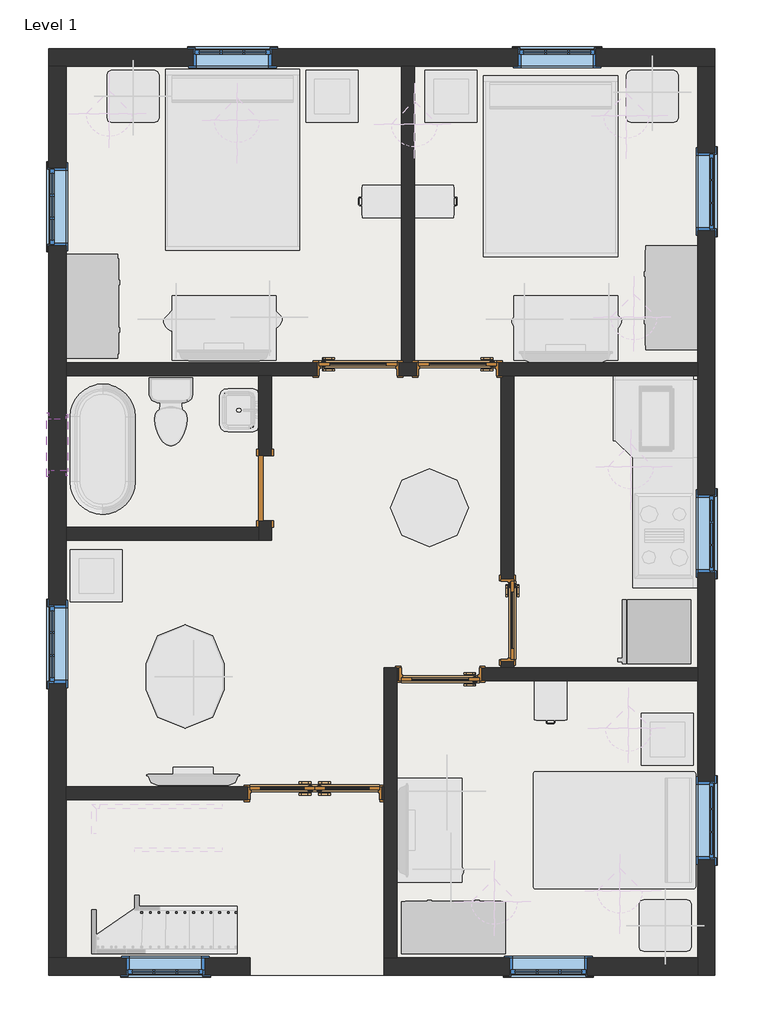
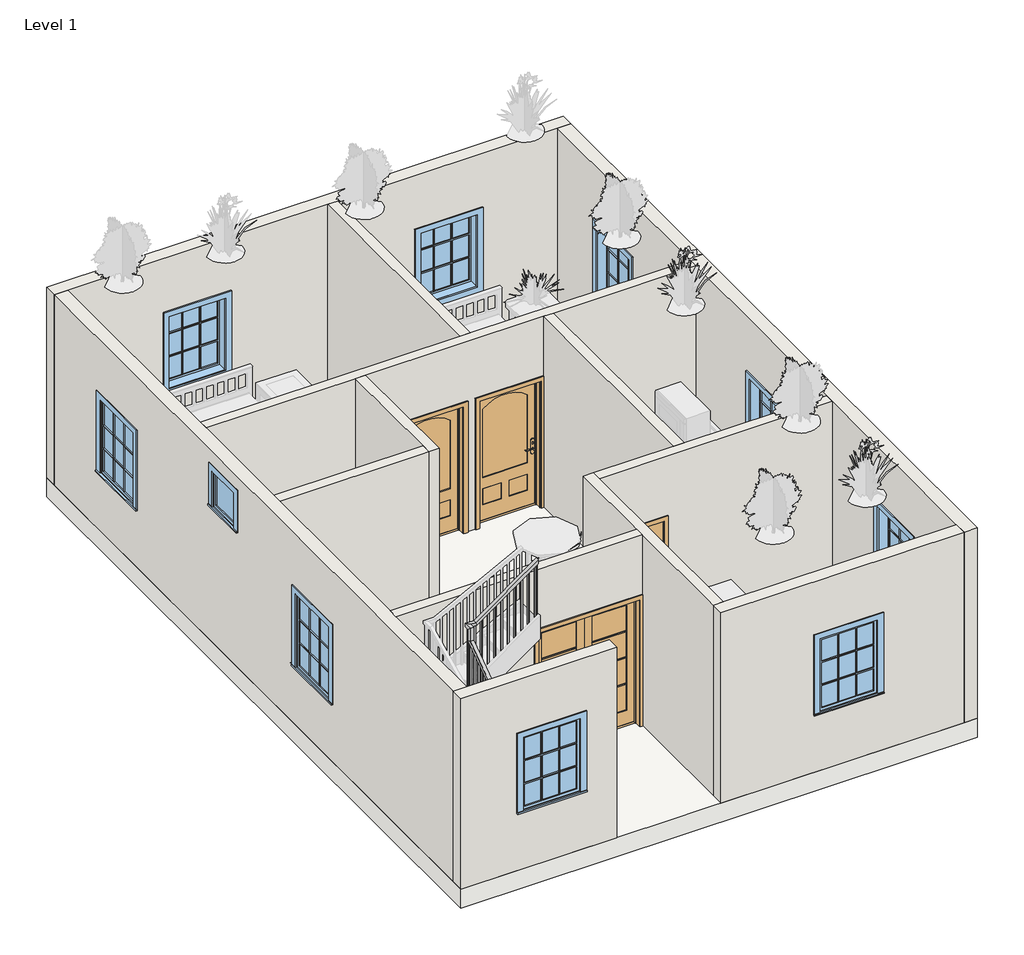
# One storey, part 1 of 2: 13 walls, 10 windows, 6 doors, 1 railing, 1 slab.
"""IFC4 building model written with IfcOpenShell, lengths in millimetres."""

from ifc_helpers import new_model, si_unit, frame, origin, origin_with_axes, place, context, project, spatial, polyline, outline, extrude, faceted_brep, transform, mapped, element, save
from components import door_5d363d20, door_808aeb8e, door_94998e6c, door_255cab33, window_29c06734, window_e41d21a6

model = new_model("IFC4")

# Units and contexts
model_context = context("Model", 3, world=origin())
ifc_project = project(units=[si_unit("LENGTHUNIT", "METRE", prefix="MILLI")], contexts=[model_context])

# Site, building, storey
site = spatial("IfcSite", under=ifc_project)
building = spatial("IfcBuilding", under=site)
storey = spatial("IfcBuildingStorey", under=building, Name="Level 1", Elevation=0.0)

# Doors
placement = place(None, origin())
door_shape = door_5d363d20(model_context)
element("IfcDoor", 1, ObjectType="36\" x 80\"", at=placement, inside=storey, context=model_context, shape_type="MappedRepresentation", body=[
    mapped(door_shape, transform((-9424.8047602, 10392.474435, 0.0), x_axis=(-1.0, 0.0, 0.0), y_axis=(0.0, -1.0, 0.0), z_axis=(0.0, 0.0, 1.0))),
])
element("IfcDoor", 2, ObjectType="36\" x 80\"", at=placement, inside=storey, context=model_context, shape_type="MappedRepresentation", body=[
    mapped(door_shape, transform((-7669.0297602, 7442.899435, 0.0), x_axis=(0.0, 1.0, 0.0), y_axis=(-1.0, 0.0, 0.0), z_axis=(0.0, 0.0, 1.0))),
])
element("IfcDoor", 3, ObjectType="36\" x 80\"", at=placement, inside=storey, context=model_context, shape_type="MappedRepresentation", body=[
    mapped(door_shape, transform((-8459.6047602, 6804.724435, 0.0), x_axis=(1.0, 0.0, 0.0), y_axis=(0.0, 1.0, 0.0), z_axis=(0.0, 0.0, 1.0))),
])
door_2_shape = door_808aeb8e(model_context)
element("IfcDoor", 4, ObjectType="36\" x 80\"", at=placement, inside=storey, context=model_context, shape_type="MappedRepresentation", body=[
    mapped(door_2_shape, transform((-8256.4047602, 10392.474435, 0.0), x_axis=(1.0, 0.0, 0.0), y_axis=(0.0, 1.0, 0.0), z_axis=(0.0, 0.0, 1.0))),
])
door_3_shape = door_94998e6c(model_context)
element("IfcDoor", 5, ObjectType="Door-Exterior-Double-Full Glass-Wood_Clad : 60\" x 80\"", at=placement, inside=storey, context=model_context, shape_type="MappedRepresentation", body=[
    mapped(door_3_shape, transform((-9932.8047602, 5414.074435, 0.0), x_axis=(1.0, 0.0, 0.0), y_axis=(0.0, 1.0, 0.0), z_axis=(0.0, 0.0, 1.0))),
])
door_4_shape = door_255cab33(model_context)
element("IfcDoor", 6, ObjectType="Single-Flush : 30\" x 80\"", at=placement, inside=storey, context=model_context, shape_type="MappedRepresentation", body=[
    mapped(door_4_shape, transform((-10517.0047602, 8992.299435, 0.0), x_axis=(0.0, -1.0, 0.0), y_axis=(1.0, 0.0, 0.0), z_axis=(0.0, 0.0, 1.0))),
])

# Railing
element("IfcRailing", 7, ObjectType="Handrail - Rectangular", at=placement, inside=storey, context=model_context, shape_type="SolidModel", body=[
    faceted_brep([(-10847.2047602, 3988.499435, 1381.9082396), (-10847.2047602, 3988.499435, 1318.3782167), (-10847.2047602, 4039.299435, 1318.3782167), (-10847.2047602, 4039.299435, 1381.9082396), (-11968.5364521, 3988.499435, 2224.0110577), (-12019.3364521, 3988.499435, 2198.6310519), (-12019.3364521, 4039.299435, 2198.6310519), (-11968.5364521, 4039.299435, 2224.0110577), (-11968.5364521, 3988.499435, 2365.3316897), (-12019.3364521, 3988.499435, 2314.5316897), (-12019.3364521, 4039.299435, 2314.5316897), (-11968.5364521, 4039.299435, 2365.3316897), (-12095.5364521, 3988.499435, 2365.3316897), (-12095.5364521, 3988.499435, 2314.5316897), (-12044.7364521, 4039.299435, 2314.5316897), (-12044.7364521, 4039.299435, 2365.3316897), (-12095.5364521, 4115.499435, 2365.3316897), (-12095.5364521, 4131.3621783, 2314.5316897), (-12044.7364521, 4131.3621783, 2314.5316897), (-12044.7364521, 4115.499435, 2365.3316897), (-12095.5364521, 4699.699435, 2769.5924376), (-12095.5364521, 4750.499435, 2742.9686812), (-12044.7364521, 4750.499435, 2742.9686812), (-12044.7364521, 4699.699435, 2769.5924376), (-12095.5364521, 4699.699435, 2979.2954752), (-12095.5364521, 4750.499435, 2928.4954752), (-12044.7364521, 4750.499435, 2928.4954752), (-12044.7364521, 4699.699435, 2979.2954752), (-12095.5364521, 4826.699435, 2979.2954752), (-12095.5364521, 4826.699435, 2928.4954752), (-12044.7364521, 4775.899435, 2928.4954752), (-12044.7364521, 4775.899435, 2979.2954752), (-11968.5364521, 4826.699435, 2979.2954752), (-11952.2655241, 4826.699435, 2928.4954752), (-11952.2655241, 4775.899435, 2928.4954752), (-11968.5364521, 4775.899435, 2979.2954752), (-11023.5532442, 4826.699435, 3653.8404346), (-11023.5532442, 4775.899435, 3653.8404346), (-11023.5532442, 4775.899435, 3591.4259716), (-11023.5532442, 4826.699435, 3591.4259716)], [[[0, 1, 2, 3]], [[1, 0, 4, 5]], [[2, 1, 5, 6]], [[3, 2, 6, 7]], [[0, 3, 7, 4]], [[5, 4, 8, 9]], [[6, 5, 9, 10]], [[7, 6, 10, 11]], [[4, 7, 11, 8]], [[9, 8, 12, 13]], [[10, 9, 13, 14]], [[11, 10, 14, 15]], [[8, 11, 15, 12]], [[13, 12, 16, 17]], [[14, 13, 17, 18]], [[15, 14, 18, 19]], [[12, 15, 19, 16]], [[17, 16, 20, 21]], [[18, 17, 21, 22]], [[19, 18, 22, 23]], [[16, 19, 23, 20]], [[21, 20, 24, 25]], [[22, 21, 25, 26]], [[23, 22, 26, 27]], [[20, 23, 27, 24]], [[25, 24, 28, 29]], [[26, 25, 29, 30]], [[27, 26, 30, 31]], [[24, 27, 31, 28]], [[29, 28, 32, 33]], [[30, 29, 33, 34]], [[31, 30, 34, 35]], [[28, 31, 35, 32]], [[36, 37, 38, 39]], [[33, 32, 36, 39]], [[34, 33, 39, 38]], [[35, 34, 38, 37]], [[32, 35, 37, 36]]]),
    extrude(outline(polyline([(3576.3942675, -11044.6114521), (3562.796056, -11063.6614521), (2540.0, -11063.6614521), (2540.0, -11044.6114521), (3576.3942675, -11044.6114521)])), frame((0.0, 4791.774435, 0.0), z_axis=(0.0, 1.0, 0.0), x_axis=(0.0, 0.0, 1.0)), (0.0, 0.0, 1.0), 19.05),
    extrude(outline(polyline([(3503.8704731, -11146.2114521), (3490.2722616, -11165.2614521), (2540.0, -11165.2614521), (2540.0, -11146.2114521), (3503.8704731, -11146.2114521)])), frame((0.0, 4791.774435, 0.0), z_axis=(0.0, 1.0, 0.0), x_axis=(0.0, 0.0, 1.0)), (0.0, 0.0, 1.0), 19.05),
    extrude(outline(polyline([(3431.3466787, -11247.8114521), (3417.7484672, -11266.8614521), (2540.0, -11266.8614521), (2540.0, -11247.8114521), (3431.3466787, -11247.8114521)])), frame((0.0, 4791.774435, 0.0), z_axis=(0.0, 1.0, 0.0), x_axis=(0.0, 0.0, 1.0)), (0.0, 0.0, 1.0), 19.05),
    extrude(outline(polyline([(3358.8228843, -11349.4114521), (3345.2246729, -11368.4614521), (2370.6666667, -11368.4614521), (2370.6666667, -11349.4114521), (3358.8228843, -11349.4114521)])), frame((0.0, 4791.774435, 0.0), z_axis=(0.0, 1.0, 0.0), x_axis=(0.0, 0.0, 1.0)), (0.0, 0.0, 1.0), 19.05),
    extrude(outline(polyline([(3286.2990899, -11451.0114521), (3272.7008785, -11470.0614521), (2370.6666667, -11470.0614521), (2370.6666667, -11451.0114521), (3286.2990899, -11451.0114521)])), frame((0.0, 4791.774435, 0.0), z_axis=(0.0, 1.0, 0.0), x_axis=(0.0, 0.0, 1.0)), (0.0, 0.0, 1.0), 19.05),
    extrude(outline(polyline([(3213.7752955, -11552.6114521), (3200.1770841, -11571.6614521), (2370.6666667, -11571.6614521), (2370.6666667, -11552.6114521), (3213.7752955, -11552.6114521)])), frame((0.0, 4791.774435, 0.0), z_axis=(0.0, 1.0, 0.0), x_axis=(0.0, 0.0, 1.0)), (0.0, 0.0, 1.0), 19.05),
    extrude(outline(polyline([(3141.2515011, -11654.2114521), (3127.6532897, -11673.2614521), (2201.3333333, -11673.2614521), (2201.3333333, -11654.2114521), (3141.2515011, -11654.2114521)])), frame((0.0, 4791.774435, 0.0), z_axis=(0.0, 1.0, 0.0), x_axis=(0.0, 0.0, 1.0)), (0.0, 0.0, 1.0), 19.05),
    extrude(outline(polyline([(3068.7277067, -11755.8114521), (3055.1294953, -11774.8614521), (2201.3333333, -11774.8614521), (2201.3333333, -11755.8114521), (3068.7277067, -11755.8114521)])), frame((0.0, 4791.774435, 0.0), z_axis=(0.0, 1.0, 0.0), x_axis=(0.0, 0.0, 1.0)), (0.0, 0.0, 1.0), 19.05),
    extrude(outline(polyline([(2996.2039123, -11857.4114521), (2982.6057009, -11876.4614521), (2032.0, -11876.4614521), (2032.0, -11857.4114521), (2996.2039123, -11857.4114521)])), frame((0.0, 4791.774435, 0.0), z_axis=(0.0, 1.0, 0.0), x_axis=(0.0, 0.0, 1.0)), (0.0, 0.0, 1.0), 19.05),
    extrude(outline(polyline([(-11978.0614521, 4791.774435), (-11978.0614521, 4810.824435), (-11959.0114521, 4810.824435), (-11959.0114521, 4791.774435), (-11978.0614521, 4791.774435)])), frame((0.0, 0.0, 2032.0), z_axis=(0.0, 0.0, 1.0), x_axis=(1.0, 0.0, 0.0)), (0.0, 0.0, 1.0), 896.4954752),
    extrude(outline(polyline([(4719.3935773, 2721.4437287), (4738.4435773, 2734.6261443), (4738.4435773, 1862.6666667), (4719.3935773, 1862.6666667), (4719.3935773, 2721.4437287)])), frame((-12079.6614521, 0.0, 0.0), z_axis=(1.0, 0.0, 0.0), x_axis=(0.0, 1.0, 0.0)), (0.0, 0.0, 1.0), 19.05),
    extrude(outline(polyline([(4617.7935773, 2651.1375116), (4636.8435773, 2664.3199273), (4636.8435773, 1693.3333333), (4617.7935773, 1693.3333333), (4617.7935773, 2651.1375116)])), frame((-12079.6614521, 0.0, 0.0), z_axis=(1.0, 0.0, 0.0), x_axis=(0.0, 1.0, 0.0)), (0.0, 0.0, 1.0), 19.05),
    extrude(outline(polyline([(4516.1935773, 2580.8312946), (4535.2435773, 2594.0137103), (4535.2435773, 1693.3333333), (4516.1935773, 1693.3333333), (4516.1935773, 2580.8312946)])), frame((-12079.6614521, 0.0, 0.0), z_axis=(1.0, 0.0, 0.0), x_axis=(0.0, 1.0, 0.0)), (0.0, 0.0, 1.0), 19.05),
    extrude(outline(polyline([(4414.5935773, 2510.5250776), (4433.6435773, 2523.7074933), (4433.6435773, 1524.0), (4414.5935773, 1524.0), (4414.5935773, 2510.5250776)])), frame((-12079.6614521, 0.0, 0.0), z_axis=(1.0, 0.0, 0.0), x_axis=(0.0, 1.0, 0.0)), (0.0, 0.0, 1.0), 19.05),
    extrude(outline(polyline([(4312.9935773, 2440.2188606), (4332.0435773, 2453.4012762), (4332.0435773, 1524.0), (4312.9935773, 1524.0), (4312.9935773, 2440.2188606)])), frame((-12079.6614521, 0.0, 0.0), z_axis=(1.0, 0.0, 0.0), x_axis=(0.0, 1.0, 0.0)), (0.0, 0.0, 1.0), 19.05),
    extrude(outline(polyline([(4211.3935773, 2369.9126435), (4230.4435773, 2383.0950592), (4230.4435773, 1524.0), (4211.3935773, 1524.0), (4211.3935773, 2369.9126435)])), frame((-12079.6614521, 0.0, 0.0), z_axis=(1.0, 0.0, 0.0), x_axis=(0.0, 1.0, 0.0)), (0.0, 0.0, 1.0), 19.05),
    extrude(outline(polyline([(4109.7935773, 2299.6064265), (4128.8435773, 2312.7888422), (4128.8435773, 1354.6666667), (4109.7935773, 1354.6666667), (4109.7935773, 2299.6064265)])), frame((-12079.6614521, 0.0, 0.0), z_axis=(1.0, 0.0, 0.0), x_axis=(0.0, 1.0, 0.0)), (0.0, 0.0, 1.0), 19.05),
    extrude(outline(polyline([(-12056.8797602, 4023.424435), (-12056.8797602, 4004.374435), (-12075.9297602, 4004.374435), (-12075.9297602, 4023.424435), (-12056.8797602, 4023.424435)])), frame((0.0, 0.0, 1354.6666667), z_axis=(0.0, 0.0, 1.0), x_axis=(1.0, 0.0, 0.0)), (0.0, 0.0, 1.0), 959.865023),
    extrude(outline(polyline([(2150.5254636, -11955.2797602), (2164.83172, -11974.3297602), (1185.3333333, -11974.3297602), (1185.3333333, -11955.2797602), (2150.5254636, -11955.2797602)])), frame((0.0, 4004.374435, 0.0), z_axis=(0.0, 1.0, 0.0), x_axis=(0.0, 0.0, 1.0)), (0.0, 0.0, 1.0), 19.05),
    extrude(outline(polyline([(2074.2254295, -11853.6797602), (2088.5316859, -11872.7297602), (1016.0, -11872.7297602), (1016.0, -11853.6797602), (2074.2254295, -11853.6797602)])), frame((0.0, 4004.374435, 0.0), z_axis=(0.0, 1.0, 0.0), x_axis=(0.0, 0.0, 1.0)), (0.0, 0.0, 1.0), 19.05),
    extrude(outline(polyline([(1997.9253954, -11752.0797602), (2012.2316518, -11771.1297602), (1016.0, -11771.1297602), (1016.0, -11752.0797602), (1997.9253954, -11752.0797602)])), frame((0.0, 4004.374435, 0.0), z_axis=(0.0, 1.0, 0.0), x_axis=(0.0, 0.0, 1.0)), (0.0, 0.0, 1.0), 19.05),
    extrude(outline(polyline([(1921.6253613, -11650.4797602), (1935.9316177, -11669.5297602), (846.6666667, -11669.5297602), (846.6666667, -11650.4797602), (1921.6253613, -11650.4797602)])), frame((0.0, 4004.374435, 0.0), z_axis=(0.0, 1.0, 0.0), x_axis=(0.0, 0.0, 1.0)), (0.0, 0.0, 1.0), 19.05),
    extrude(outline(polyline([(1845.3253272, -11548.8797602), (1859.6315836, -11567.9297602), (846.6666667, -11567.9297602), (846.6666667, -11548.8797602), (1845.3253272, -11548.8797602)])), frame((0.0, 4004.374435, 0.0), z_axis=(0.0, 1.0, 0.0), x_axis=(0.0, 0.0, 1.0)), (0.0, 0.0, 1.0), 19.05),
    extrude(outline(polyline([(1769.0252931, -11447.2797602), (1783.3315495, -11466.3297602), (846.6666667, -11466.3297602), (846.6666667, -11447.2797602), (1769.0252931, -11447.2797602)])), frame((0.0, 4004.374435, 0.0), z_axis=(0.0, 1.0, 0.0), x_axis=(0.0, 0.0, 1.0)), (0.0, 0.0, 1.0), 19.05),
    extrude(outline(polyline([(1692.725259, -11345.6797602), (1707.0315154, -11364.7297602), (677.3333333, -11364.7297602), (677.3333333, -11345.6797602), (1692.725259, -11345.6797602)])), frame((0.0, 4004.374435, 0.0), z_axis=(0.0, 1.0, 0.0), x_axis=(0.0, 0.0, 1.0)), (0.0, 0.0, 1.0), 19.05),
    extrude(outline(polyline([(1616.4252249, -11244.0797602), (1630.7314813, -11263.1297602), (677.3333333, -11263.1297602), (677.3333333, -11244.0797602), (1616.4252249, -11244.0797602)])), frame((0.0, 4004.374435, 0.0), z_axis=(0.0, 1.0, 0.0), x_axis=(0.0, 0.0, 1.0)), (0.0, 0.0, 1.0), 19.05),
    extrude(outline(polyline([(1540.1251908, -11142.4797602), (1554.4314472, -11161.5297602), (677.3333333, -11161.5297602), (677.3333333, -11142.4797602), (1540.1251908, -11142.4797602)])), frame((0.0, 4004.374435, 0.0), z_axis=(0.0, 1.0, 0.0), x_axis=(0.0, 0.0, 1.0)), (0.0, 0.0, 1.0), 19.05),
    extrude(outline(polyline([(1463.8251567, -11040.8797602), (1478.1314131, -11059.9297602), (508.0, -11059.9297602), (508.0, -11040.8797602), (1463.8251567, -11040.8797602)])), frame((0.0, 4004.374435, 0.0), z_axis=(0.0, 1.0, 0.0), x_axis=(0.0, 0.0, 1.0)), (0.0, 0.0, 1.0), 19.05),
    extrude(outline(polyline([(1387.5251226, -10939.2797602), (1401.831379, -10958.3297602), (508.0, -10958.3297602), (508.0, -10939.2797602), (1387.5251226, -10939.2797602)])), frame((0.0, 4004.374435, 0.0), z_axis=(0.0, 1.0, 0.0), x_axis=(0.0, 0.0, 1.0)), (0.0, 0.0, 1.0), 19.05),
    extrude(outline(polyline([(-12079.6614521, 4791.774435), (-12079.6614521, 4810.824435), (-12060.6114521, 4810.824435), (-12060.6114521, 4791.774435), (-12079.6614521, 4791.774435)])), frame((0.0, 0.0, 1862.6666667), z_axis=(0.0, 0.0, 1.0), x_axis=(1.0, 0.0, 0.0)), (0.0, 0.0, 1.0), 1065.8288085),
    extrude(outline(polyline([(-12060.6114521, 4008.1935773), (-12079.6614521, 4008.1935773), (-12079.6614521, 4027.2435773), (-12060.6114521, 4027.2435773), (-12060.6114521, 4008.1935773)])), frame((0.0, 0.0, 1354.6666667), z_axis=(0.0, 0.0, 1.0), x_axis=(1.0, 0.0, 0.0)), (0.0, 0.0, 1.0), 959.865023),
    extrude(outline(polyline([(-12060.6114521, 4023.424435), (-12060.6114521, 4004.374435), (-12079.6614521, 4004.374435), (-12079.6614521, 4023.424435), (-12060.6114521, 4023.424435)])), frame((0.0, 0.0, 1354.6666667), z_axis=(0.0, 0.0, 1.0), x_axis=(1.0, 0.0, 0.0)), (0.0, 0.0, 1.0), 959.865023),
    extrude(outline(polyline([(-12057.0923258, 4023.424435), (-12057.0923258, 4004.374435), (-12076.1423258, 4004.374435), (-12076.1423258, 4023.424435), (-12057.0923258, 4023.424435)])), frame((0.0, 0.0, 1354.6666667), z_axis=(0.0, 0.0, 1.0), x_axis=(1.0, 0.0, 0.0)), (0.0, 0.0, 1.0), 959.865023),
    extrude(outline(polyline([(3591.4259716, -11023.5532442), (3577.8277602, -11042.6032442), (2540.0, -11042.6032442), (2540.0, -11023.5532442), (3591.4259716, -11023.5532442)])), frame((0.0, 4791.774435, 0.0), z_axis=(0.0, 1.0, 0.0), x_axis=(0.0, 0.0, 1.0)), (0.0, 0.0, 1.0), 19.05),
    extrude(outline(polyline([(1318.3782167, -10847.2047602), (1332.6844731, -10866.2547602), (508.0, -10866.2547602), (508.0, -10847.2047602), (1318.3782167, -10847.2047602)])), frame((0.0, 4004.374435, 0.0), z_axis=(0.0, 1.0, 0.0), x_axis=(0.0, 0.0, 1.0)), (0.0, 0.0, 1.0), 19.05),
])

# Slab
element("IfcSlab", 8, ObjectType="Generic - 12\"", at=placement, inside=storey, context=model_context, shape_type="SweptSolid", body=[
    extrude(outline(polyline([(-5233.8047602, 14148.499435), (-5233.8047602, 3277.299435), (-13057.0047602, 3277.299435), (-13057.0047602, 14148.499435), (-5233.8047602, 14148.499435)])), frame((0.0, 0.0, -304.8), z_axis=(0.0, 0.0, 1.0), x_axis=(1.0, 0.0, 0.0)), (0.0, 0.0, 1.0), 304.8),
])

# Walls
element("IfcWall", 9, ObjectType="Generic - 8\"", at=placement, inside=storey, context=model_context, shape_type="Brep", body=[
    faceted_brep([(-13057.0047602, 13945.299435, 0.0), (-12853.8047602, 13945.299435, 0.0), (-8916.8047602, 13945.299435, 0.0), (-8764.4047602, 13945.299435, 0.0), (-5437.0047602, 13945.299435, 0.0), (-5233.8047602, 13945.299435, 0.0), (-5233.8047602, 13945.299435, 3048.0), (-5437.0047602, 13945.299435, 3048.0), (-8764.4047602, 13945.299435, 3048.0), (-8916.8047602, 13945.299435, 3048.0), (-12853.8047602, 13945.299435, 3048.0), (-13057.0047602, 13945.299435, 3048.0), (-10440.8047602, 13945.299435, 2133.6), (-10440.8047602, 13945.299435, 914.4), (-11355.2047602, 13945.299435, 914.4), (-11355.2047602, 13945.299435, 2133.6), (-6630.8047602, 13945.299435, 2133.6), (-6630.8047602, 13945.299435, 914.4), (-7545.2047602, 13945.299435, 914.4), (-7545.2047602, 13945.299435, 2133.6), (-13057.0047602, 14148.499435, 0.0), (-13057.0047602, 14148.499435, 3048.0), (-5233.8047602, 14148.499435, 3048.0), (-5233.8047602, 14148.499435, 0.0), (-10440.8047602, 14148.499435, 2133.6), (-11355.2047602, 14148.499435, 2133.6), (-11355.2047602, 14148.499435, 914.4), (-10440.8047602, 14148.499435, 914.4), (-6630.8047602, 14148.499435, 2133.6), (-7545.2047602, 14148.499435, 2133.6), (-7545.2047602, 14148.499435, 914.4), (-6630.8047602, 14148.499435, 914.4)], [[[0, 1, 2, 3, 4, 5, 6, 7, 8, 9, 10, 11], [12, 13, 14, 15], [16, 17, 18, 19]], [[20, 21, 22, 23], [24, 25, 26, 27], [28, 29, 30, 31]], [[5, 4, 3, 2, 1, 0, 20, 23]], [[6, 5, 23, 22]], [[0, 11, 21, 20]], [[13, 12, 24, 27]], [[14, 13, 27, 26]], [[15, 14, 26, 25]], [[12, 15, 25, 24]], [[17, 16, 28, 31]], [[18, 17, 31, 30]], [[19, 18, 30, 29]], [[16, 19, 29, 28]], [[11, 10, 9, 8, 7, 6, 22, 21]]]),
])
element("IfcWall", 10, ObjectType="Generic - 8\"", at=placement, inside=storey, context=model_context, shape_type="Brep", body=[
    faceted_brep([(-5437.0047602, 13945.299435, 0.0), (-5437.0047602, 10465.499435, 0.0), (-5437.0047602, 10313.099435, 0.0), (-5437.0047602, 6884.099435, 0.0), (-5437.0047602, 6731.699435, 0.0), (-5437.0047602, 3480.499435, 0.0), (-5437.0047602, 3277.299435, 0.0), (-5437.0047602, 3277.299435, 3048.0), (-5437.0047602, 3480.499435, 3048.0), (-5437.0047602, 6731.699435, 3048.0), (-5437.0047602, 6884.099435, 3048.0), (-5437.0047602, 10313.099435, 3048.0), (-5437.0047602, 10465.499435, 3048.0), (-5437.0047602, 13945.299435, 3048.0), (-5437.0047602, 12014.899435, 2133.6), (-5437.0047602, 12014.899435, 914.4), (-5437.0047602, 12929.299435, 914.4), (-5437.0047602, 12929.299435, 2133.6), (-5437.0047602, 8001.699435, 2133.6), (-5437.0047602, 8001.699435, 914.4), (-5437.0047602, 8916.099435, 914.4), (-5437.0047602, 8916.099435, 2133.6), (-5437.0047602, 4636.199435, 2133.6), (-5437.0047602, 4636.199435, 914.4), (-5437.0047602, 5550.599435, 914.4), (-5437.0047602, 5550.599435, 2133.6), (-5233.8047602, 13945.299435, 0.0), (-5233.8047602, 13945.299435, 3048.0), (-5233.8047602, 3277.299435, 3048.0), (-5233.8047602, 3277.299435, 0.0), (-5233.8047602, 12014.899435, 2133.6), (-5233.8047602, 12929.299435, 2133.6), (-5233.8047602, 12929.299435, 914.4), (-5233.8047602, 12014.899435, 914.4), (-5233.8047602, 8001.699435, 2133.6), (-5233.8047602, 8916.099435, 2133.6), (-5233.8047602, 8916.099435, 914.4), (-5233.8047602, 8001.699435, 914.4), (-5233.8047602, 4636.199435, 2133.6), (-5233.8047602, 5550.599435, 2133.6), (-5233.8047602, 5550.599435, 914.4), (-5233.8047602, 4636.199435, 914.4)], [[[0, 1, 2, 3, 4, 5, 6, 7, 8, 9, 10, 11, 12, 13], [14, 15, 16, 17], [18, 19, 20, 21], [22, 23, 24, 25]], [[26, 27, 28, 29], [30, 31, 32, 33], [34, 35, 36, 37], [38, 39, 40, 41]], [[6, 5, 4, 3, 2, 1, 0, 26, 29]], [[0, 13, 27, 26]], [[7, 6, 29, 28]], [[15, 14, 30, 33]], [[16, 15, 33, 32]], [[17, 16, 32, 31]], [[14, 17, 31, 30]], [[19, 18, 34, 37]], [[20, 19, 37, 36]], [[21, 20, 36, 35]], [[18, 21, 35, 34]], [[23, 22, 38, 41]], [[24, 23, 41, 40]], [[25, 24, 40, 39]], [[22, 25, 39, 38]], [[13, 12, 11, 10, 9, 8, 7, 28, 27]]]),
])
element("IfcWall", 11, ObjectType="Generic - 8\"", at=placement, inside=storey, context=model_context, shape_type="Brep", body=[
    faceted_brep([(-5437.0047602, 3480.499435, 0.0), (-8967.6047602, 3480.499435, 0.0), (-9120.0047602, 3480.499435, 0.0), (-9120.0047602, 3480.499435, 3048.0), (-8967.6047602, 3480.499435, 3048.0), (-5437.0047602, 3480.499435, 3048.0), (-7646.8047602, 3480.499435, 2133.6), (-7646.8047602, 3480.499435, 914.4), (-6732.4047602, 3480.499435, 914.4), (-6732.4047602, 3480.499435, 2133.6), (-5437.0047602, 3277.299435, 0.0), (-5437.0047602, 3277.299435, 3048.0), (-9120.0047602, 3277.299435, 3048.0), (-9120.0047602, 3277.299435, 0.0), (-7646.8047602, 3277.299435, 2133.6), (-6732.4047602, 3277.299435, 2133.6), (-6732.4047602, 3277.299435, 914.4), (-7646.8047602, 3277.299435, 914.4)], [[[0, 1, 2, 3, 4, 5], [6, 7, 8, 9]], [[10, 11, 12, 13], [14, 15, 16, 17]], [[2, 1, 0, 10, 13]], [[0, 5, 11, 10]], [[7, 6, 14, 17]], [[8, 7, 17, 16]], [[9, 8, 16, 15]], [[6, 9, 15, 14]], [[3, 2, 13, 12]], [[5, 4, 3, 12, 11]]]),
])
element("IfcWall", 12, ObjectType="Generic - 8\"", at=placement, inside=storey, context=model_context, shape_type="Brep", body=[
    faceted_brep([(-12853.8047602, 3480.499435, 0.0), (-12853.8047602, 5334.699435, 0.0), (-12853.8047602, 5487.099435, 0.0), (-12853.8047602, 8382.699435, 0.0), (-12853.8047602, 8535.099435, 0.0), (-12853.8047602, 10313.099435, 0.0), (-12853.8047602, 10465.499435, 0.0), (-12853.8047602, 13945.299435, 0.0), (-12853.8047602, 13945.299435, 3048.0), (-12853.8047602, 10465.499435, 3048.0), (-12853.8047602, 10313.099435, 3048.0), (-12853.8047602, 8535.099435, 3048.0), (-12853.8047602, 8382.699435, 3048.0), (-12853.8047602, 5487.099435, 3048.0), (-12853.8047602, 5334.699435, 3048.0), (-12853.8047602, 3480.499435, 3048.0), (-12853.8047602, 12751.499435, 2133.6), (-12853.8047602, 12751.499435, 914.4), (-12853.8047602, 11837.099435, 914.4), (-12853.8047602, 11837.099435, 2133.6), (-12853.8047602, 7620.699435, 2133.6), (-12853.8047602, 7620.699435, 914.4), (-12853.8047602, 6706.299435, 914.4), (-12853.8047602, 6706.299435, 2133.6), (-12853.8047602, 9805.099435, 2768.6), (-12853.8047602, 9805.099435, 2159.0), (-12853.8047602, 9195.499435, 2159.0), (-12853.8047602, 9195.499435, 2768.6), (-13057.0047602, 3480.499435, 0.0), (-13057.0047602, 3480.499435, 3048.0), (-13057.0047602, 13945.299435, 3048.0), (-13057.0047602, 13945.299435, 0.0), (-13057.0047602, 12751.499435, 2133.6), (-13057.0047602, 11837.099435, 2133.6), (-13057.0047602, 11837.099435, 914.4), (-13057.0047602, 12751.499435, 914.4), (-13057.0047602, 7620.699435, 2133.6), (-13057.0047602, 6706.299435, 2133.6), (-13057.0047602, 6706.299435, 914.4), (-13057.0047602, 7620.699435, 914.4), (-13057.0047602, 9805.099435, 2768.6), (-13057.0047602, 9195.499435, 2768.6), (-13057.0047602, 9195.499435, 2159.0), (-13057.0047602, 9805.099435, 2159.0)], [[[0, 1, 2, 3, 4, 5, 6, 7, 8, 9, 10, 11, 12, 13, 14, 15], [16, 17, 18, 19], [20, 21, 22, 23], [24, 25, 26, 27]], [[28, 29, 30, 31], [32, 33, 34, 35], [36, 37, 38, 39], [40, 41, 42, 43]], [[7, 6, 5, 4, 3, 2, 1, 0, 28, 31]], [[8, 7, 31, 30]], [[0, 15, 29, 28]], [[17, 16, 32, 35]], [[18, 17, 35, 34]], [[19, 18, 34, 33]], [[16, 19, 33, 32]], [[21, 20, 36, 39]], [[22, 21, 39, 38]], [[23, 22, 38, 37]], [[20, 23, 37, 36]], [[25, 24, 40, 43]], [[26, 25, 43, 42]], [[27, 26, 42, 41]], [[24, 27, 41, 40]], [[15, 14, 13, 12, 11, 10, 9, 8, 30, 29]]]),
])
element("IfcWall", 13, ObjectType="Generic - 8\"", at=placement, inside=storey, context=model_context, shape_type="Brep", body=[
    faceted_brep([(-10694.8047602, 3480.499435, 0.0), (-12853.8047602, 3480.499435, 0.0), (-13057.0047602, 3480.499435, 0.0), (-13057.0047602, 3480.499435, 3048.0), (-12853.8047602, 3480.499435, 3048.0), (-10694.8047602, 3480.499435, 3048.0), (-12142.6047602, 3480.499435, 2133.6), (-12142.6047602, 3480.499435, 914.4), (-11228.2047602, 3480.499435, 914.4), (-11228.2047602, 3480.499435, 2133.6), (-10694.8047602, 3277.299435, 0.0), (-10694.8047602, 3277.299435, 3048.0), (-13057.0047602, 3277.299435, 3048.0), (-13057.0047602, 3277.299435, 0.0), (-12142.6047602, 3277.299435, 2133.6), (-11228.2047602, 3277.299435, 2133.6), (-11228.2047602, 3277.299435, 914.4), (-12142.6047602, 3277.299435, 914.4)], [[[0, 1, 2, 3, 4, 5], [6, 7, 8, 9]], [[10, 11, 12, 13], [14, 15, 16, 17]], [[2, 1, 0, 10, 13]], [[0, 5, 11, 10]], [[3, 2, 13, 12]], [[6, 9, 15, 14]], [[9, 8, 16, 15]], [[8, 7, 17, 16]], [[7, 6, 14, 17]], [[5, 4, 3, 12, 11]]]),
])
element("IfcWall", 14, ObjectType="INNER 6\"", at=placement, inside=storey, context=model_context, shape_type="SweptSolid", body=[
    extrude(outline(polyline([(-8916.8047602, 10465.499435), (-8916.8047602, 13945.299435), (-8764.4047602, 13945.299435), (-8764.4047602, 10465.499435), (-8916.8047602, 10465.499435)])), origin_with_axes(), (0.0, 0.0, 1.0), 3048.0),
])
element("IfcWall", 15, ObjectType="INNER 6\"", at=placement, inside=storey, context=model_context, shape_type="Brep", body=[
    faceted_brep([(-12853.8047602, 10465.499435, 0.0), (-12853.8047602, 10465.499435, 3048.0), (-8916.8047602, 10465.499435, 3048.0), (-8764.4047602, 10465.499435, 3048.0), (-5437.0047602, 10465.499435, 3048.0), (-5437.0047602, 10465.499435, 0.0), (-7773.8047602, 10465.499435, 0.0), (-7773.8047602, 10465.499435, 2057.4), (-8739.0047602, 10465.499435, 2057.4), (-8739.0047602, 10465.499435, 0.0), (-8764.4047602, 10465.499435, 0.0), (-8916.8047602, 10465.499435, 0.0), (-8942.2047602, 10465.499435, 0.0), (-8942.2047602, 10465.499435, 2057.4), (-9907.4047602, 10465.499435, 2057.4), (-9907.4047602, 10465.499435, 0.0), (-12853.8047602, 10313.099435, 3048.0), (-12853.8047602, 10313.099435, 0.0), (-10593.2047602, 10313.099435, 0.0), (-10440.8047602, 10313.099435, 0.0), (-9907.4047602, 10313.099435, 0.0), (-9907.4047602, 10313.099435, 2057.4), (-8942.2047602, 10313.099435, 2057.4), (-8942.2047602, 10313.099435, 0.0), (-8739.0047602, 10313.099435, 0.0), (-8739.0047602, 10313.099435, 2057.4), (-7773.8047602, 10313.099435, 2057.4), (-7773.8047602, 10313.099435, 0.0), (-7748.4047602, 10313.099435, 0.0), (-7596.0047602, 10313.099435, 0.0), (-5437.0047602, 10313.099435, 0.0), (-5437.0047602, 10313.099435, 3048.0), (-7596.0047602, 10313.099435, 3048.0), (-7748.4047602, 10313.099435, 3048.0), (-10440.8047602, 10313.099435, 3048.0), (-10593.2047602, 10313.099435, 3048.0)], [[[0, 1, 2, 3, 4, 5, 6, 7, 8, 9, 10, 11, 12, 13, 14, 15]], [[16, 17, 18, 19, 20, 21, 22, 23, 24, 25, 26, 27, 28, 29, 30, 31, 32, 33, 34, 35]], [[17, 0, 15, 20, 19, 18]], [[5, 30, 29, 28, 27, 6]], [[23, 12, 11, 10, 9, 24]], [[1, 0, 17, 16]], [[5, 4, 31, 30]], [[14, 21, 20, 15]], [[21, 14, 13, 22]], [[22, 13, 12, 23]], [[26, 7, 6, 27]], [[7, 26, 25, 8]], [[8, 25, 24, 9]], [[4, 3, 2, 1, 16, 35, 34, 33, 32, 31]]]),
])
element("IfcWall", 16, ObjectType="INNER 6\"", at=placement, inside=storey, context=model_context, shape_type="Brep", body=[
    faceted_brep([(-10593.2047602, 8611.299435, 2032.0), (-10593.2047602, 8611.299435, 0.0), (-10593.2047602, 8535.099435, 0.0), (-10593.2047602, 8382.699435, 0.0), (-10593.2047602, 8382.699435, 3048.0), (-10593.2047602, 8535.099435, 3048.0), (-10593.2047602, 10313.099435, 3048.0), (-10593.2047602, 10313.099435, 0.0), (-10593.2047602, 9373.299435, 0.0), (-10593.2047602, 9373.299435, 2032.0), (-10440.8047602, 8382.699435, 0.0), (-10440.8047602, 8611.299435, 0.0), (-10440.8047602, 8611.299435, 2032.0), (-10440.8047602, 9373.299435, 2032.0), (-10440.8047602, 9373.299435, 0.0), (-10440.8047602, 10313.099435, 0.0), (-10440.8047602, 10313.099435, 3048.0), (-10440.8047602, 8382.699435, 3048.0)], [[[0, 1, 2, 3, 4, 5, 6, 7, 8, 9]], [[10, 11, 12, 13, 14, 15, 16, 17]], [[8, 7, 15, 14]], [[3, 2, 1, 11, 10]], [[7, 6, 16, 15]], [[4, 3, 10, 17]], [[12, 11, 1, 0]], [[13, 12, 0, 9]], [[14, 13, 9, 8]], [[6, 5, 4, 17, 16]]]),
])
element("IfcWall", 17, ObjectType="INNER 6\"", at=placement, inside=storey, context=model_context, shape_type="SweptSolid", body=[
    extrude(outline(polyline([(-12853.8047602, 8535.099435), (-10593.2047602, 8535.099435), (-10593.2047602, 8382.699435), (-12853.8047602, 8382.699435), (-12853.8047602, 8535.099435)])), origin_with_axes(), (0.0, 0.0, 1.0), 3048.0),
])
element("IfcWall", 18, ObjectType="INNER 6\"", at=placement, inside=storey, context=model_context, shape_type="SweptSolid", body=[
    extrude(outline(polyline([(3048.0, -12853.8047602), (0.0, -12853.8047602), (0.0, -10720.2047602), (2057.4, -10720.2047602), (2057.4, -9145.4047602), (0.0, -9145.4047602), (0.0, -9120.0047602), (3048.0, -9120.0047602), (3048.0, -12853.8047602)])), frame((0.0, 5334.699435, 0.0), z_axis=(0.0, 1.0, 0.0), x_axis=(0.0, 0.0, 1.0)), (0.0, 0.0, 1.0), 152.4),
])
element("IfcWall", 19, ObjectType="INNER 6\"", at=placement, inside=storey, context=model_context, shape_type="Brep", body=[
    faceted_brep([(-9120.0047602, 6884.099435, 0.0), (-9120.0047602, 5487.099435, 0.0), (-9120.0047602, 5334.699435, 0.0), (-9120.0047602, 3480.499435, 0.0), (-9120.0047602, 3480.499435, 3048.0), (-9120.0047602, 5334.699435, 3048.0), (-9120.0047602, 5487.099435, 3048.0), (-9120.0047602, 6884.099435, 3048.0), (-8967.6047602, 6884.099435, 0.0), (-8967.6047602, 6884.099435, 3048.0), (-8967.6047602, 6731.699435, 3048.0), (-8967.6047602, 3480.499435, 3048.0), (-8967.6047602, 3480.499435, 0.0), (-8967.6047602, 6731.699435, 0.0)], [[[0, 1, 2, 3, 4, 5, 6, 7]], [[8, 9, 10, 11, 12, 13]], [[3, 2, 1, 0, 8, 13, 12]], [[4, 3, 12, 11]], [[0, 7, 9, 8]], [[7, 6, 5, 4, 11, 10, 9]]]),
])
element("IfcWall", 20, ObjectType="INNER 6\"", at=placement, inside=storey, context=model_context, shape_type="Brep", body=[
    faceted_brep([(-8967.6047602, 6731.699435, 3048.0), (-8967.6047602, 6731.699435, 0.0), (-8942.2047602, 6731.699435, 0.0), (-8942.2047602, 6731.699435, 2057.4), (-7977.0047602, 6731.699435, 2057.4), (-7977.0047602, 6731.699435, 0.0), (-5437.0047602, 6731.699435, 0.0), (-5437.0047602, 6731.699435, 3048.0), (-8967.6047602, 6884.099435, 0.0), (-8967.6047602, 6884.099435, 3048.0), (-7748.4047602, 6884.099435, 3048.0), (-7596.0047602, 6884.099435, 3048.0), (-5437.0047602, 6884.099435, 3048.0), (-5437.0047602, 6884.099435, 0.0), (-7596.0047602, 6884.099435, 0.0), (-7748.4047602, 6884.099435, 0.0), (-7977.0047602, 6884.099435, 0.0), (-7977.0047602, 6884.099435, 2057.4), (-8942.2047602, 6884.099435, 2057.4), (-8942.2047602, 6884.099435, 0.0)], [[[0, 1, 2, 3, 4, 5, 6, 7]], [[8, 9, 10, 11, 12, 13, 14, 15, 16, 17, 18, 19]], [[1, 8, 19, 2]], [[13, 6, 5, 16, 15, 14]], [[1, 0, 9, 8]], [[7, 6, 13, 12]], [[4, 17, 16, 5]], [[17, 4, 3, 18]], [[18, 3, 2, 19]], [[0, 7, 12, 11, 10, 9]]]),
])
element("IfcWall", 21, ObjectType="INNER 6\"", at=placement, inside=storey, context=model_context, shape_type="SweptSolid", body=[
    extrude(outline(polyline([(6884.099435, 0.0), (6884.099435, 3048.0), (10313.099435, 3048.0), (10313.099435, 0.0), (7925.499435, 0.0), (7925.499435, 2057.4), (6960.299435, 2057.4), (6960.299435, 0.0), (6884.099435, 0.0)])), frame((-7748.4047602, 0.0, 0.0), z_axis=(1.0, 0.0, 0.0), x_axis=(0.0, 1.0, 0.0)), (0.0, 0.0, 1.0), 152.4),
])

# Windows
window_shape = window_29c06734(model_context)
element("IfcWindow", 22, ObjectType="Casement 3x3 with Trim : 36\" x 48\"", at=placement, inside=storey, context=model_context, shape_type="MappedRepresentation", body=[
    mapped(window_shape, transform((-10898.0047602, 14046.899435, 0.0), x_axis=(1.0, 0.0, 0.0), y_axis=(0.0, 1.0, 0.0), z_axis=(0.0, 0.0, 1.0))),
])
element("IfcWindow", 23, ObjectType="Casement 3x3 with Trim : 36\" x 48\"", at=placement, inside=storey, context=model_context, shape_type="MappedRepresentation", body=[
    mapped(window_shape, transform((-12955.4047602, 12294.299435, 0.0), x_axis=(0.0, 1.0, 0.0), y_axis=(-1.0, 0.0, 0.0), z_axis=(0.0, 0.0, 1.0))),
])
element("IfcWindow", 24, ObjectType="Casement 3x3 with Trim : 36\" x 48\"", at=placement, inside=storey, context=model_context, shape_type="MappedRepresentation", body=[
    mapped(window_shape, transform((-7088.0047602, 14046.899435, 0.0), x_axis=(1.0, 0.0, 0.0), y_axis=(0.0, 1.0, 0.0), z_axis=(0.0, 0.0, 1.0))),
])
element("IfcWindow", 25, ObjectType="Casement 3x3 with Trim : 36\" x 48\"", at=placement, inside=storey, context=model_context, shape_type="MappedRepresentation", body=[
    mapped(window_shape, transform((-5335.4047602, 12472.099435, 0.0), x_axis=(0.0, -1.0, 0.0), y_axis=(1.0, 0.0, 0.0), z_axis=(0.0, 0.0, 1.0))),
])
element("IfcWindow", 26, ObjectType="Casement 3x3 with Trim : 36\" x 48\"", at=placement, inside=storey, context=model_context, shape_type="MappedRepresentation", body=[
    mapped(window_shape, transform((-5335.4047602, 8458.899435, 0.0), x_axis=(0.0, -1.0, 0.0), y_axis=(1.0, 0.0, 0.0), z_axis=(0.0, 0.0, 1.0))),
])
element("IfcWindow", 27, ObjectType="Casement 3x3 with Trim : 36\" x 48\"", at=placement, inside=storey, context=model_context, shape_type="MappedRepresentation", body=[
    mapped(window_shape, transform((-5335.4047602, 5093.399435, 0.0), x_axis=(0.0, -1.0, 0.0), y_axis=(1.0, 0.0, 0.0), z_axis=(0.0, 0.0, 1.0))),
])
element("IfcWindow", 28, ObjectType="Casement 3x3 with Trim : 36\" x 48\"", at=placement, inside=storey, context=model_context, shape_type="MappedRepresentation", body=[
    mapped(window_shape, transform((-7189.6047602, 3378.899435, 0.0), x_axis=(-1.0, 0.0, 0.0), y_axis=(0.0, -1.0, 0.0), z_axis=(0.0, 0.0, 1.0))),
])
element("IfcWindow", 29, ObjectType="Casement 3x3 with Trim : 36\" x 48\"", at=placement, inside=storey, context=model_context, shape_type="MappedRepresentation", body=[
    mapped(window_shape, transform((-11685.4047602, 3378.899435, 0.0), x_axis=(-1.0, 0.0, 0.0), y_axis=(0.0, -1.0, 0.0), z_axis=(0.0, 0.0, 1.0))),
])
element("IfcWindow", 30, ObjectType="Casement 3x3 with Trim : 36\" x 48\"", at=placement, inside=storey, context=model_context, shape_type="MappedRepresentation", body=[
    mapped(window_shape, transform((-12955.4047602, 7163.499435, 0.0), x_axis=(0.0, 1.0, 0.0), y_axis=(-1.0, 0.0, 0.0), z_axis=(0.0, 0.0, 1.0))),
])
window_2_shape = window_e41d21a6(model_context)
element("IfcWindow", 31, ObjectType="Transom with Trim : 24\" x 24\"", at=placement, inside=storey, context=model_context, shape_type="MappedRepresentation", body=[
    mapped(window_2_shape, transform((-12955.4047602, 9538.399435, 0.0), x_axis=(0.0, 1.0, 0.0), y_axis=(-1.0, 0.0, 0.0), z_axis=(0.0, 0.0, 1.0))),
])

save(model, "model.ifc")

# Revit data of these elements
# Type "36\" x 80\""
#   Type Mark = "8"
#   Assembly Code = "B2030100"
#   Analytic Construction = "French door, wood frame with single glass"
#   Threshold Offset [instance default] = 0' - 0 1/2"
#   Thickness = 0' - 1 3/8"
#   Thermal Resistance (R) = 1.0696 (h·ft²·°F)/BTU
#   Swing Angle [instance default] = 90.00°
#   Stiles = 0' - 4 3/4"
#   Rough Width = 3' - 2"
#   Rough Height = 6' - 9"
#   Radius = 1' - 8.05625"
#   Lock Rail = 0' - 7 1/8"
#   Height = 6' - 8"
#   Width = 3' - 0"
#   Heat Transfer Coefficient (U) = 0.9350 BTU/(h·ft²·°F)
#   Door Offset [instance default] = 0' - 0"
#   Bottom Rail = 0' - 9 1/2"
#   Threshold [instance default] = yes
#   Function = 1
#   Exterior Trim [instance default] = yes
#   Trim Material = Cherry
#   Threshold Material = Cherry
#   Panel Material = Cherry
#   Glazing = Glass
#   Frame Material = Cherry
#   Door Handle Material = Aluminum
#   Visual Light Transmittance = 0
#   Solar Heat Gain Coefficient = 0
#   Wall Closure = (empty or 0)
#   Construction Type = (empty or 0)
# Type "Door-Exterior-Double-Full Glass-Wood_Clad : 60\" x 80\""
#   Type Mark = "9"
#   Assembly Code = "B2030100"
#   Analytic Construction = "French door, wood frame with double glass"
#   Top Rail = 0' - 4 11/16"
#   Threshold Offset [instance default] = 0' - 0 1/2"
#   Thickness = 0' - 1 3/8"
#   Thermal Resistance (R) = 1.9158 (h·ft²·°F)/BTU
#   Swing Angle [instance default] = 90.00°
#   Stiles = 0' - 4 3/4"
#   Rough Width = 5' - 2"
#   Rough Height = 6' - 9"
#   Panel Width = 2' - 6"
#   Door Offset [instance default] = 0' - 0"
#   Height = 6' - 8"
#   Width = 5' - 0"
#   Heat Transfer Coefficient (U) = 0.5220 BTU/(h·ft²·°F)
#   Bottom Rail = 0' - 9 1/8"
#   Exterior Trim [instance default] = yes
#   Threshold [instance default] = yes
#   Show Grill [instance default] = yes
#   Function = 1
#   Trim Material = Cherry
#   Threshold Material = Cherry
#   Panel Material = Cherry
#   Glazing = Glass
#   Frame Material = Cherry
#   Door Handle Material = Aluminum
#   Visual Light Transmittance = 0
#   Solar Heat Gain Coefficient = 0
#   Wall Closure = (empty or 0)
#   Construction Type = (empty or 0)
# Type "Single-Flush : 30\" x 80\""
#   Type Mark = "5"
#   Construction Type Id = "MDOOR"
#   Assembly Code = "C1020"
#   Analytic Construction = "Metal"
#   Thickness = 0' - 2"
#   Heat Transfer Coefficient (U) = 0.651978 BTU/(h·ft²·°F)
#   Height = 6' - 8"
#   Trim Projection Ext = 0' - 1"
#   Trim Projection Int = 0' - 1"
#   Trim Width = 0' - 3"
#   Width = 2' - 6"
#   Define Thermal Properties by = 1
#   Door Material = Door - Panel
#   Frame Material = Door - Frame
#   Visual Light Transmittance = 0
#   Solar Heat Gain Coefficient = 0
#   Function = (empty or 0)
#   Wall Closure = (empty or 0)
# Type "Handrail - Rectangular"
#   Assembly Code = "C2010400"
#   built-in parameter 1008612 = 0.0416667 (stored number, unit not read)
#   built-in parameter 1008611 = 0.0416667 (stored number, unit not read)
#   built-in parameter 1008609 = 0.333333 (stored number, unit not read)
#   built-in parameter 1008604 = 0.166667 (stored number, unit not read)
#   built-in parameter 1008603 = 0.166667 (stored number, unit not read)
#   Railing Height = 3' - 0"
#   built-in parameter 1008630 = 2
#   built-in parameter 1008610 = 2
#   built-in parameter 1008618 = Baluster - Square : 3/4"
# Type "Generic - 12\""
#   Assembly Code = "B1010"
#   Function = 0
#   Layers, outside or top first: 1' - 0" no material (function 1)
# Type "Generic - 8\""
#   Assembly Code = "B2010"
#   Layers, outside or top first: 0' - 8" "Brick, Common" (function 1)
# Type "INNER 6\""
#   Assembly Code = "B2010"
#   Layers, outside or top first: 0' - 6" "Brick, Common" (function 1)
# Type "Casement 3x3 with Trim : 36\" x 48\""
#   Type Mark = "10"
#   Construction Type Id = "GSP4R"
#   Assembly Code = "B2020100"
#   Analytic Construction = "1/8 in Pilkington single glazing"
#   Visual Light Transmittance = 0.9
#   Solar Heat Gain Coefficient = 0.78
#   Heat Transfer Coefficient (U) = 0.6496 BTU/(h·ft²·°F)
#   Height = 4' - 0"
#   Default Sill Height = 3' - 0"
#   Trim Projection - Ext. = 0' - 0 1/2"
#   Trim Projection - Int. = 0' - 0 3/4"
#   Trim Width - Exterior = 0' - 3 1/2"
#   Trim Width - Interior = 0' - 3 1/2"
#   Width = 3' - 0"
#   Window Inset = 0' - 0 3/4"
#   Define Thermal Properties by = 1
#   Glass Pane Material = Glass
#   Sash Material = Sash
#   Trim Exterior Material = Trim
#   Trim Interior Material = Trim
#   Wall Closure = (empty or 0)
# Type "Transom with Trim : 24\" x 24\""
#   Type Mark = "13"
#   Construction Type Id = "GSP4R"
#   Assembly Code = "B2020100"
#   Analytic Construction = "1/8 in Pilkington single glazing"
#   Visual Light Transmittance = 0.9
#   Solar Heat Gain Coefficient = 0.78
#   Heat Transfer Coefficient (U) = 0.6496 BTU/(h·ft²·°F)
#   Height = 2' - 0"
#   Default Sill Height = 7' - 1"
#   Trim Projection - Ext. = 0' - 0 1/2"
#   Trim Projection - Int. = 0' - 0 3/4"
#   Trim Width - Exterior = 0' - 3 1/2"
#   Trim Width - Interior = 0' - 3 1/2"
#   Width = 2' - 0"
#   Window Inset = 0' - 0 3/4"
#   Define Thermal Properties by = 1
#   Glass Pane Material = Glass
#   Sash Material = Sash
#   Trim Exterior Material = Trim
#   Trim Interior Material = Trim
#   Wall Closure = (empty or 0)
# Elements 1, 2, 3, 4 (IfcDoor, "36\" x 80\"")
#   Threshold Offset = 0' - 0 1/2"
#   Swing Angle = 90.00°
#   Door Offset = 0' - 0"
#   Threshold = yes
#   Exterior Trim = yes
#   Phase Created = New Construction
#   Materials on its faces: "Cherry", "Aluminum", "Glass"
# Element 5 (IfcDoor, "Door-Exterior-Double-Full Glass-Wood_Clad : 60\" x 80\"")
#   Threshold Offset = 0' - 0 1/2"
#   Swing Angle = 90.00°
#   Door Offset = 0' - 0"
#   Threshold = yes
#   Show Grill = yes
#   Exterior Trim = yes
#   Phase Created = New Construction
#   Materials on its faces: "Cherry", "Aluminum", "Glass"
# Element 6 (IfcDoor, "Single-Flush : 30\" x 80\"")
#   Phase Created = New Construction
#   Materials on its faces: "Door - Frame", "Door - Panel"
# Element 7 (IfcRailing, "Handrail - Rectangular")
#   Phase Created = New Construction
# Element 8 (IfcSlab, "Generic - 12\"")
#   Height Offset From Level = 0' - 0"
#   Phase Created = New Construction
#   Materials on its faces: "Default Floor"
# Elements 9, 10, 11, 12, 13 (IfcWall, "Generic - 8\"")
#   Top Offset = 0' - 0"
#   Base Offset = 0' - 0"
#   Unconnected Height = 10' - 0"
#   wall height = 10' - 0"
#   Phase Created = New Construction
#   Base Constraint = Level 1
#   Materials on its faces: "Brick, Common"
# Elements 14, 15, 16, 17, 18, 19, 20, 21 (IfcWall, "INNER 6\"")
#   Top Offset = 0' - 0"
#   Base Offset = 0' - 0"
#   Unconnected Height = 10' - 0"
#   wall height = 10' - 0"
#   Phase Created = New Construction
#   Base Constraint = Level 1
#   Materials on its faces: "Brick, Common"
# Element 22 (IfcWindow, "Casement 3x3 with Trim : 36\" x 48\"")
#   Mark = "1"
#   Phase Created = New Construction
#   Materials on its faces: "Sash", "Glass", "Trim"
# Element 23 (IfcWindow, "Casement 3x3 with Trim : 36\" x 48\"")
#   Mark = "2"
#   Phase Created = New Construction
#   Materials on its faces: "Sash", "Glass", "Trim"
# Element 24 (IfcWindow, "Casement 3x3 with Trim : 36\" x 48\"")
#   Mark = "3"
#   Phase Created = New Construction
#   Materials on its faces: "Sash", "Glass", "Trim"
# Element 25 (IfcWindow, "Casement 3x3 with Trim : 36\" x 48\"")
#   Mark = "4"
#   Phase Created = New Construction
#   Materials on its faces: "Sash", "Glass", "Trim"
# Element 26 (IfcWindow, "Casement 3x3 with Trim : 36\" x 48\"")
#   Mark = "5"
#   Phase Created = New Construction
#   Materials on its faces: "Sash", "Glass", "Trim"
# Element 27 (IfcWindow, "Casement 3x3 with Trim : 36\" x 48\"")
#   Mark = "6"
#   Phase Created = New Construction
#   Materials on its faces: "Sash", "Glass", "Trim"
# Element 28 (IfcWindow, "Casement 3x3 with Trim : 36\" x 48\"")
#   Mark = "7"
#   Phase Created = New Construction
#   Materials on its faces: "Sash", "Glass", "Trim"
# Element 29 (IfcWindow, "Casement 3x3 with Trim : 36\" x 48\"")
#   Mark = "8"
#   Phase Created = New Construction
#   Materials on its faces: "Sash", "Glass", "Trim"
# Element 30 (IfcWindow, "Casement 3x3 with Trim : 36\" x 48\"")
#   Mark = "9"
#   Phase Created = New Construction
#   Materials on its faces: "Sash", "Glass", "Trim"
# Element 31 (IfcWindow, "Transom with Trim : 24\" x 24\"")
#   Mark = "10"
#   Phase Created = New Construction
#   Materials on its faces: "Sash", "Trim", "Glass"
# Materials
#   "Cherry": class "Wood", colour RGB 226 177 128, transparency 0, Description = "Prunus Serotina", Cost = 0
#   "Glass": class "Glass", colour RGB 0 128 192, transparency 0.75, Description = "Soda Lime Glass", Cost = 0
#   "Aluminum": class "Metal", colour RGB 247 247 247, transparency 0, Description = "Aluminum 6061", Cost = 0
#   "Door - Panel": class "Wood", colour RGB 210 159 95, transparency 0
#   "Door - Frame": colour RGB 118 70 51, transparency 0
#   "Brick, Common": class "Masonry", colour RGB 170 98 104, transparency 0, Description = "Common brick", Cost = 0
#   "Sash": class "Wood", colour RGB 224 178 126, transparency 0
#   "Trim": class "Wood", colour RGB 224 178 126, transparency 0
#   "Default Floor": colour RGB 128 128 128, transparency 0
# Room at (-10885.4, 12200.985) mm, phase "New Construction", upper level "Level 1", upper offset 10' - 0", lower offset 0' - 0"
#   Number = "1"
#   Name = "BEDROOM-1"
# Room at (-6994.611, 12021.622) mm, phase "New Construction", upper level "Level 1", upper offset 10' - 0", lower offset 0' - 0"
#   Number = "2"
#   Name = "BEDROOM-2"
# Room at (-11694.996, 9093.007) mm, phase "New Construction", upper level "Level 1", upper offset 10' - 0", lower offset 0' - 0"
#   Number = "3"
#   Name = "TOILET"
# Room at (-6532.877, 8367.376) mm, phase "New Construction", upper level "Level 1", upper offset 10' - 0", lower offset 0' - 0"
#   Number = "4"
#   Name = "KITCHEN"
# Room at (-9866.196, 7830.852) mm, phase "New Construction", upper level "Level 1", upper offset 10' - 0", lower offset 0' - 0"
#   Number = "6"
#   Name = "LIVING/DINING"
# Room at (-11694.996, 6778.785) mm, phase "New Construction", upper level "Level 1", upper offset 10' - 0", lower offset 0' - 0"
#   Number = "5"
#   Name = "Room"
